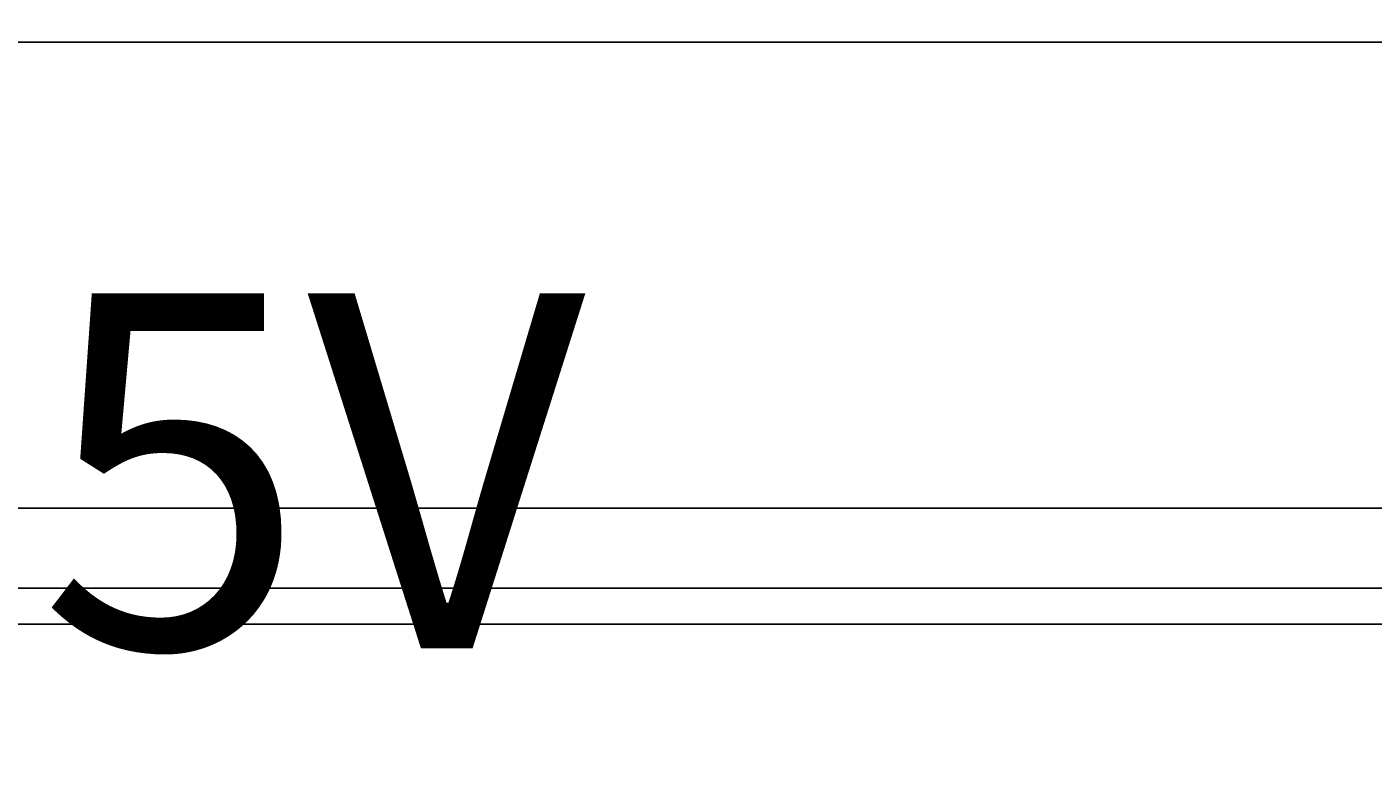
# Model space of a CAD drawing. Units: inches. Extents: x 35362 to 73946, y 43607 to 67532.
# Tile 70 of 134: x 48464 to 49302, y 48798 to 49269. Entities that reach past the tile are written whole.
import ezdxf

# ---------------------------------------------------------------- set-up
doc = ezdxf.new("R2010")
doc.units = ezdxf.units.IN
doc.header["$MEASUREMENT"] = 0
doc.layers.add('A-ANNO-DIMS', color=2, linetype='Continuous', lineweight=18)
doc.layers.add('E-ANNO-TEXT', color=5, linetype='Continuous', lineweight=18)
doc.styles.get("Standard").update_dxf_attribs({"font": 'arial.ttf'})
doc.dimstyles.get("Standard").update_dxf_attribs({"dimtxt": 0.18, "dimasz": 0.18, "dimexe": 0.18, "dimexo": 0.0625, "dimgap": 0.09, "dimtad": 0, "dimtih": 1, "dimtoh": 1, "dimdec": 4, "dimzin": 0, "dimdsep": 46, "dimtxsty": 'Standard', "dimcen": 0.09, "dimadec": 0, "dimazin": 0, "dimtfac": 1, "dimtdec": 4, "dimtofl": 0, "dimtmove": 0, "dimatfit": 3, "dimfxl": 1, "dimtolj": 1, "dimtzin": 0, "dimarcsym": 0})

# ---------------------------------------------------------------- blocks, each defined once
blk = doc.blocks.new('*D11')
at = {"layer": 'A-ANNO-DIMS', "color": 0, "lineweight": -2, "transparency": 16777216}
for p, q in [((47978.66, 56028.77), (47978.66, 43606.68)), ((53109.76, 56028.77), (53109.76, 43606.68)), ((47978.84, 43606.86), (50543.87, 43606.86)), ((53109.58, 43606.86), (50544.55, 43606.86))]:
    blk.add_line(p, q, dxfattribs=at)
at = {"layer": 'A-ANNO-DIMS', "color": 0, "transparency": 16777216}
for points in [[(47978.84, 43606.89), (47978.84, 43606.83), (47978.66, 43606.86)], [(53109.58, 43606.89), (53109.58, 43606.83), (53109.76, 43606.86)]]:
    blk.add_solid(points, dxfattribs=at)
at = {"layer": 'Defpoints', "color": 0, "transparency": 16777216}
for p in [(47978.66, 56028.84), (53109.76, 56028.84), (53109.76, 43606.86)]:
    blk.add_point(p, dxfattribs=at)
at = {"layer": 'A-ANNO-DIMS', "color": 0, "transparency": 16777216, "insert": (50544.21, 43606.86), "char_height": 0.18, "attachment_point": 5}
blk.add_mtext('\\A1;5131', dxfattribs=at)
blk = doc.blocks.new('*D13')
at = {"layer": 'A-ANNO-DIMS', "color": 0, "lineweight": -2, "transparency": 16777216}
for p, q in [((48373.49, 51694.02), (48373.49, 43606.68)), ((51029.04, 51694.02), (51029.04, 43606.68)), ((48373.67, 43606.86), (49700.8, 43606.86)), ((51028.86, 43606.86), (49701.73, 43606.86))]:
    blk.add_line(p, q, dxfattribs=at)
at = {"layer": 'A-ANNO-DIMS', "color": 0, "transparency": 16777216}
for points in [[(48373.67, 43606.89), (48373.67, 43606.83), (48373.49, 43606.86)], [(51028.86, 43606.89), (51028.86, 43606.83), (51029.04, 43606.86)]]:
    blk.add_solid(points, dxfattribs=at)
at = {"layer": 'Defpoints', "color": 0, "transparency": 16777216}
for p in [(48373.49, 51694.09), (51029.04, 51694.09), (51029.04, 43606.86)]:
    blk.add_point(p, dxfattribs=at)
at = {"layer": 'A-ANNO-DIMS', "color": 0, "transparency": 16777216, "insert": (49701.27, 43606.86), "char_height": 0.18, "attachment_point": 5}
blk.add_mtext('\\A1;2655.6', dxfattribs=at)
blk = doc.blocks.new('*D67')
at = {"layer": 'A-ANNO-DIMS', "color": 0, "lineweight": -2, "transparency": 16777216}
for p, q in [((56873.54, 53351.53), (35361.77, 53351.53)), ((35361.95, 53351.35), (35361.95, 49400.89)), ((35361.95, 45450.07), (35361.95, 49400.53)), ((53793.58, 45449.89), (35361.77, 45449.89))]:
    blk.add_line(p, q, dxfattribs=at)
at = {"layer": 'A-ANNO-DIMS', "color": 0, "transparency": 16777216}
for points in [[(35361.92, 53351.35), (35361.98, 53351.35), (35361.95, 53351.53)], [(35361.92, 45450.07), (35361.98, 45450.07), (35361.95, 45449.89)]]:
    blk.add_solid(points, dxfattribs=at)
at = {"layer": 'Defpoints', "color": 0, "transparency": 16777216}
for p in [(35361.95, 53351.53), (56873.6, 53351.53), (53793.64, 45449.89)]:
    blk.add_point(p, dxfattribs=at)
at = {"layer": 'A-ANNO-DIMS', "color": 0, "transparency": 16777216, "insert": (35361.95, 49400.71), "char_height": 0.18, "attachment_point": 5}
blk.add_mtext('\\A1;7901.6', dxfattribs=at)
blk = doc.blocks.new('*D84')
at = {"layer": 'A-ANNO-DIMS', "color": 0, "lineweight": -2, "transparency": 16777216}
for p, q in [((55540.23, 49259.94), (35361.77, 49259.94)), ((35361.95, 49259.76), (35361.95, 49115.14)), ((35361.95, 48970.16), (35361.95, 49114.78)), ((55540.23, 48969.98), (35361.77, 48969.98))]:
    blk.add_line(p, q, dxfattribs=at)
at = {"layer": 'A-ANNO-DIMS', "color": 0, "transparency": 16777216}
for points in [[(35361.92, 49259.76), (35361.98, 49259.76), (35361.95, 49259.94)], [(35361.92, 48970.16), (35361.98, 48970.16), (35361.95, 48969.98)]]:
    blk.add_solid(points, dxfattribs=at)
at = {"layer": 'Defpoints', "color": 0, "transparency": 16777216}
for p in [(35361.95, 49259.94), (55540.3, 49259.94), (55540.3, 48969.98)]:
    blk.add_point(p, dxfattribs=at)
at = {"layer": 'A-ANNO-DIMS', "color": 0, "transparency": 16777216, "insert": (35361.95, 49114.96), "char_height": 0.18, "attachment_point": 5}
blk.add_mtext('\\A1;289.96', dxfattribs=at)
blk = doc.blocks.new('*D86')
at = {"layer": 'A-ANNO-DIMS', "color": 0, "lineweight": -2, "transparency": 16777216}
for p, q in [((51285.53, 49320.08), (35361.77, 49320.08)), ((35361.95, 49319.9), (35361.95, 49120.26)), ((35361.95, 48920.26), (35361.95, 49119.9)), ((51285.53, 48920.08), (35361.77, 48920.08))]:
    blk.add_line(p, q, dxfattribs=at)
at = {"layer": 'A-ANNO-DIMS', "color": 0, "transparency": 16777216}
for points in [[(35361.92, 49319.9), (35361.98, 49319.9), (35361.95, 49320.08)], [(35361.92, 48920.26), (35361.98, 48920.26), (35361.95, 48920.08)]]:
    blk.add_solid(points, dxfattribs=at)
at = {"layer": 'Defpoints', "color": 0, "transparency": 16777216}
for p in [(35361.95, 49320.08), (51285.59, 49320.08), (51285.59, 48920.08)]:
    blk.add_point(p, dxfattribs=at)
at = {"layer": 'A-ANNO-DIMS', "color": 0, "transparency": 16777216, "insert": (35361.95, 49120.08), "char_height": 0.18, "attachment_point": 5}
blk.add_mtext('\\A1;400.0', dxfattribs=at)
blk = doc.blocks.new('*D89')
at = {"layer": 'A-ANNO-DIMS', "color": 0, "lineweight": -2, "transparency": 16777216}
for p, q in [((53707.72, 48897.74), (35361.77, 48897.74)), ((35361.95, 48897.56), (35361.95, 48303.16)), ((35361.95, 47708.4), (35361.95, 48302.8)), ((53707.72, 47708.22), (35361.77, 47708.22))]:
    blk.add_line(p, q, dxfattribs=at)
at = {"layer": 'A-ANNO-DIMS', "color": 0, "transparency": 16777216}
for points in [[(35361.92, 48897.56), (35361.98, 48897.56), (35361.95, 48897.74)], [(35361.92, 47708.4), (35361.98, 47708.4), (35361.95, 47708.22)]]:
    blk.add_solid(points, dxfattribs=at)
at = {"layer": 'Defpoints', "color": 0, "transparency": 16777216}
for p in [(53707.78, 48897.74), (35361.95, 47708.22), (53707.78, 47708.22)]:
    blk.add_point(p, dxfattribs=at)
at = {"layer": 'A-ANNO-DIMS', "color": 0, "transparency": 16777216, "insert": (35361.95, 48302.98), "char_height": 0.18, "attachment_point": 5}
blk.add_mtext('\\A1;1189.5', dxfattribs=at)

msp = doc.modelspace()

# ---------------------------------------------------------------- texts
at = {"layer": 'E-ANNO-TEXT'}
msp.add_text('5V', height=220.866, dxfattribs=at).set_placement((48471.313, 48882.809))

# ---------------------------------------------------------------- dimensions: what is measured, and where the dimension line sits
at = {"layer": 'A-ANNO-DIMS'}
for base, p1, p2, override, picture, middle in [((53109.76, 43606.859), (47978.665, 56028.836), (53109.76, 56028.836), {"dimdec": 0, "dimlfac": 1, "dimrnd": 0, "dimzin": 0, "dimdsep": 46, "dimlunit": 2}, '*D11', (50544.212, 43606.859)), ((51029.043, 43606.859), (48373.492, 51694.087), (51029.043, 51694.087), {"dimdec": 1, "dimlfac": 1, "dimrnd": 0, "dimzin": 0, "dimdsep": 46, "dimlunit": 2}, '*D13', (49701.267, 43606.859))]:
    dim = msp.add_linear_dim(base=base, p1=p1, p2=p2, dimstyle='Standard', override=override, dxfattribs=at)
    dim.commit()
    dim.dimension.update_dxf_attribs({"geometry": picture, "text_midpoint": middle})
for base, p1, p2, override, picture, middle in [((35361.949, 53351.529), (53793.638, 45449.894), (56873.602, 53351.529), {"dimdec": 1, "dimlfac": 1, "dimrnd": 0, "dimzin": 0, "dimdsep": 46, "dimlunit": 2}, '*D67', (35361.949, 49400.712)), ((35361.949, 49320.079), (51285.595, 48920.079), (51285.595, 49320.079), {"dimdec": 1, "dimlfac": 1, "dimrnd": 0, "dimzin": 0, "dimdsep": 46, "dimlunit": 2}, '*D86', (35361.949, 49120.079)), ((35361.9491, 49259.9353), (55540.2972, 48969.9796), (55540.2972, 49259.9353), {"dimdec": 2, "dimlfac": 1, "dimrnd": 0, "dimzin": 0, "dimdsep": 46, "dimlunit": 2}, '*D84', (35361.9491, 49114.9575)), ((35361.949, 47708.216), (53707.781, 48897.738), (53707.781, 47708.216), {"dimdec": 1, "dimlfac": 1, "dimrnd": 0, "dimzin": 0, "dimdsep": 46, "dimlunit": 2}, '*D89', (35361.949, 48302.977))]:
    dim = msp.add_linear_dim(base=base, p1=p1, p2=p2, angle=90, dimstyle='Standard', override=override, dxfattribs=at)
    dim.commit()
    dim.dimension.update_dxf_attribs({"geometry": picture, "text_midpoint": middle})

doc.saveas('drawing.dxf')
